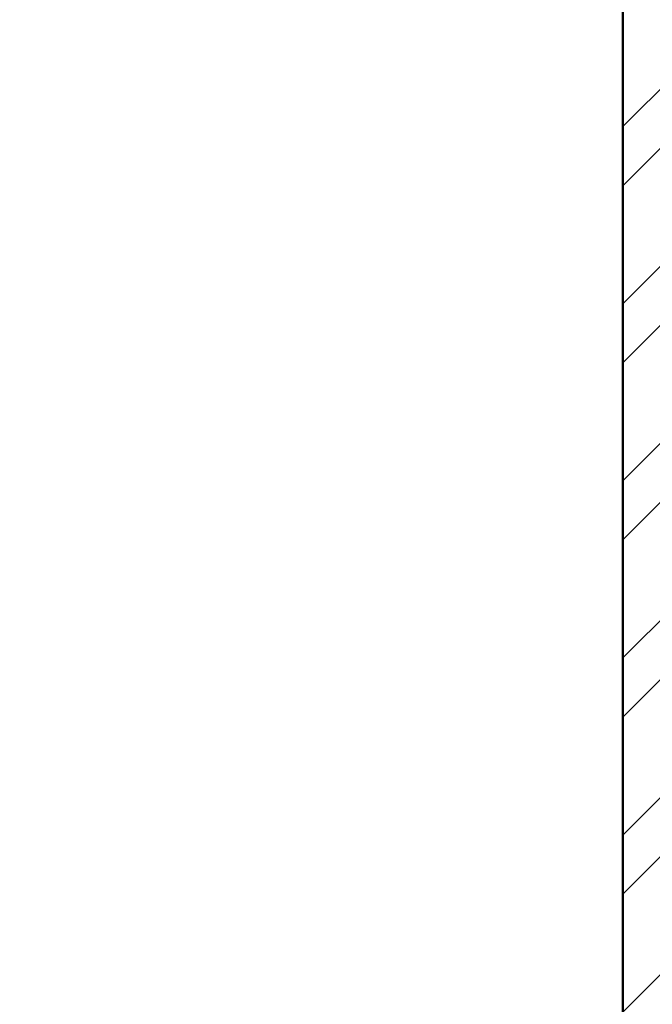
# Model space of a CAD drawing. Units: inches. Extents: x 1901 to 2863, y 888 to 2433.
# Tile 61 of 91: x 2121 to 2169, y 2127 to 2202. Entities that reach past the tile are written whole.
import ezdxf

# ---------------------------------------------------------------- set-up
doc = ezdxf.new("R2010")
doc.units = ezdxf.units.IN
doc.layers.add('A-WALL', color=7, linetype='Continuous', lineweight=50)
doc.layers.add('A-WALL-PATT', color=8, linetype='Continuous', lineweight=13)

msp = doc.modelspace()

# ---------------------------------------------------------------- hatches: boundary and pattern name
at = {"layer": 'A-WALL-PATT'}
h = msp.add_hatch(dxfattribs=at)
h.set_pattern_fill('ANSI32', color=256)
h.paths.add_polyline_path([(2192.501, 2274.134), (2141.264, 2274.134), (2141.264, 2269.634), (2192.501, 2269.634)])
h.paths.add_polyline_path([(2259.926, 2274.134), (2216.501, 2274.134), (2216.501, 2269.634), (2255.426, 2269.634), (2255.426, 2214.634), (2250.809, 2214.634), (2250.809, 2210.134), (2259.926, 2210.134), (2259.926, 2215.134), (2271.756, 2215.134), (2271.756, 2217.384), (2271.756, 2219.634), (2259.926, 2219.634)])
h.paths.add_polyline_path([(2171.426, 2269.634), (2166.926, 2269.634), (2166.926, 2219.634), (2121.238, 2219.634), (2121.238, 2215.134), (2166.926, 2215.134), (2166.926, 2083.134), (2161.807, 2083.134), (2161.807, 2078.634), (2171.426, 2078.634), (2176.996, 2078.634), (2176.996, 2080.884), (2176.996, 2083.134), (2171.426, 2083.134), (2171.426, 2210.134), (2230.912, 2210.134), (2230.912, 2212.384), (2230.912, 2214.634), (2171.426, 2214.634)])
h.paths.add_polyline_path([(2117.264, 2274.134), (2089.426, 2274.134), (2089.426, 2219.634), (2081.136, 2219.634), (2081.136, 2215.134), (2089.426, 2215.134), (2098.004, 2215.134), (2098.004, 2217.384), (2098.004, 2219.634), (2093.926, 2219.634), (2093.926, 2269.634), (2117.264, 2269.634), (2117.264, 2271.884)])
h.paths.add_polyline_path([(2343.426, 2219.634), (2329.295, 2219.634), (2329.295, 2215.134), (2338.926, 2215.134), (2338.926, 2184.739), (2343.426, 2184.739)])
h.paths.add_polyline_path([(2338.926, 2083.134), (2329.295, 2083.134), (2208.966, 2083.134), (2208.966, 2078.634), (2338.926, 2078.634)])
h.paths.add_polyline_path([(2343.426, 2136.739), (2338.926, 2136.739), (2338.926, 1872.634), (2343.426, 1872.634)])
h.paths.add_polyline_path([(2343.426, 1863.634), (2397.68, 1863.634), (2397.68, 1821.634), (2384.138, 1821.634), (2384.138, 1812.634), (2418.33, 1812.634), (2418.33, 1817.134), (2418.33, 1821.634), (2406.68, 1821.634), (2406.68, 1863.634), (2459.499, 1863.634), (2459.499, 1821.634), (2447.138, 1821.634), (2447.138, 1812.634), (2459.499, 1812.634), (2468.499, 1812.634), (2468.499, 1872.634), (2394.426, 1872.634), (2334.426, 1872.634), (2334.426, 1812.634), (2343.426, 1812.634), (2353.251, 1812.634), (2353.251, 1821.634), (2343.426, 1821.634)])
h.paths.add_polyline_path([(2510.014, 1872.634), (2468.499, 1872.634), (2468.499, 1868.134), (2510.014, 1868.134)])
h.paths.add_polyline_path([(2514.009, 1817.134), (2468.499, 1817.134), (2468.499, 1812.634), (2482.114, 1812.634), (2482.114, 1800.606), (2486.614, 1800.606), (2486.614, 1812.634), (2514.009, 1812.634)])
h.paths.add_polyline_path([(2299.247, 1814.884), (2299.247, 1817.134), (2295.926, 1817.134), (2295.926, 1854.169), (2293.676, 1854.169), (2291.426, 1854.169), (2291.426, 1817.134), (2266.109, 1817.134), (2266.109, 1812.634), (2299.247, 1812.634)])
h.paths.add_polyline_path([(2218.109, 1817.134), (2206.46, 1817.134), (2171.426, 1817.134), (2171.426, 1949.134), (2190.1, 1949.134), (2190.1, 1953.634), (2163.468, 1953.634), (2163.468, 1949.134), (2166.926, 1949.134), (2166.926, 1817.134), (2114.297, 1817.134), (2114.297, 1812.634), (2218.109, 1812.634)])
h.paths.add_polyline_path([(2029.426, 1970.922), (2024.926, 1970.922), (2024.926, 1912.717), (2029.426, 1912.717)])
h.paths.add_polyline_path([(2132.297, 1953.634), (2113.926, 1953.634), (2113.926, 1975.888), (2111.676, 1975.888), (2109.426, 1975.888), (2109.426, 1953.634), (2029.426, 1953.634), (2029.426, 1949.134), (2132.297, 1949.134)])
h.paths.add_polyline_path([(2029.426, 1853.606), (2029.31, 1853.606), (2029.31, 1853.606), (2029.426, 1853.606), (2029.426, 1864.717), (2024.926, 1864.717), (2024.926, 1812.634), (2066.297, 1812.634), (2066.297, 1814.884), (2066.297, 1817.134), (2029.426, 1817.134)])
h.paths.add_polyline_path([(2122.926, 2010.088), (2120.676, 2010.088), (2118.426, 2010.088), (2118.426, 2006.134), (2029.426, 2006.134), (2029.426, 2001.634), (2109.426, 2001.634), (2109.426, 1998.041), (2113.926, 1998.041), (2113.926, 2001.634), (2122.926, 2001.634)])
h.paths.add_polyline_path([(2029.426, 2031.376), (2024.926, 2031.376), (2024.926, 1994.922), (2027.176, 1994.922), (2029.426, 1994.922)])
h.paths.add_polyline_path([(2029.426, 2136.739), (2024.926, 2136.739), (2024.926, 2067.376), (2027.176, 2067.376), (2029.426, 2067.376)])
h.paths.add_polyline_path([(2125.618, 2083.134), (2029.426, 2083.134), (2029.426, 2078.634), (2118.426, 2078.634), (2118.426, 2030.715), (2122.926, 2030.715), (2122.926, 2078.634), (2125.618, 2078.634)])
h.paths.add_polyline_path([(2029.426, 2215.134), (2040.468, 2215.134), (2040.468, 2217.384), (2040.468, 2219.634), (2024.926, 2219.634), (2024.926, 2184.739), (2029.426, 2184.739), (2029.426, 2187.778)])
h.paths.add_polyline_path([(2686.426, 2274.134), (2659.284, 2274.134), (2659.284, 2269.634), (2681.926, 2269.634), (2681.926, 2219.634), (2676.816, 2219.634), (2676.816, 2215.134), (2681.926, 2215.134), (2697.011, 2215.134), (2697.011, 2217.384), (2697.011, 2219.634), (2686.426, 2219.634)])
h.paths.add_polyline_path([(2609.926, 2269.634), (2635.284, 2269.634), (2635.284, 2274.134), (2571.431, 2274.134), (2571.431, 2269.634), (2605.426, 2269.634), (2605.426, 2214.634), (2549.098, 2214.634), (2549.098, 2210.134), (2605.426, 2210.134), (2605.426, 2083.134), (2601.014, 2083.134), (2601.014, 2080.884), (2601.014, 2078.634), (2609.926, 2078.634), (2616.162, 2078.634), (2616.162, 2080.884), (2616.162, 2083.134), (2609.926, 2083.134), (2609.926, 2215.134), (2651.465, 2215.134), (2651.465, 2217.384), (2651.465, 2219.634), (2609.926, 2219.634)])
h.paths.add_polyline_path([(2521.426, 2269.634), (2547.431, 2269.634), (2547.431, 2271.884), (2547.431, 2274.134), (2516.926, 2274.134), (2516.926, 2219.634), (2506.41, 2219.634), (2506.41, 2215.134), (2516.926, 2215.134), (2516.926, 2210.134), (2525.402, 2210.134), (2525.402, 2212.384), (2525.402, 2214.634), (2521.426, 2214.634)])
h.paths.add_polyline_path([(2456.011, 2219.634), (2439.426, 2219.634), (2439.426, 2187.888), (2443.926, 2187.888), (2443.926, 2215.134), (2456.011, 2215.134)])
h.paths.add_polyline_path([(2752.926, 2219.634), (2739.485, 2219.634), (2739.485, 2215.134), (2748.426, 2215.134), (2748.426, 2187.888), (2752.926, 2187.888)])
h.paths.add_polyline_path([(2752.926, 2139.888), (2748.426, 2139.888), (2748.426, 2083.134), (2648.416, 2083.134), (2648.416, 2078.634), (2654.926, 2078.634), (2654.926, 2039.437), (2659.426, 2039.437), (2659.426, 2078.634), (2748.426, 2078.634), (2748.426, 2063.429), (2752.926, 2063.429)])
h.paths.add_polyline_path([(2752.926, 2010.634), (2659.426, 2010.634), (2659.426, 2015.652), (2654.926, 2015.652), (2654.926, 2010.634), (2605.426, 2010.634), (2605.426, 1920.967), (2609.926, 1920.967), (2609.926, 2006.134), (2748.426, 2006.134), (2748.426, 1982.466), (2752.926, 1982.466)])
h.paths.add_polyline_path([(2752.926, 2027.429), (2748.426, 2027.429), (2748.426, 2010.634), (2752.926, 2010.634)])
h.paths.add_polyline_path([(2748.426, 1886.134), (2609.926, 1886.134), (2609.926, 1889.719), (2605.426, 1889.719), (2605.426, 1861.262), (2609.926, 1861.262), (2609.926, 1881.634), (2748.426, 1881.634)])
h.paths.add_polyline_path([(2456.855, 2228.831), (2498.401, 2228.831), (2498.401, 2247.488), (2456.855, 2247.488)], flags=9)
h.paths.add_polyline_path([(2038.602, 2237.418), (2080.174, 2237.418), (2080.174, 2256.075), (2038.602, 2256.075)], flags=9)
h.paths.add_polyline_path([(2292.009, 1062.394), (2539.932, 1062.394), (2539.932, 1099.487), (2292.009, 1099.487)], flags=9)
h.paths.add_polyline_path([(2424.91, 1832.253), (2448.513, 1832.253), (2448.513, 1846.678), (2424.91, 1846.678)], flags=25)
h.paths.add_polyline_path([(2359.076, 1832.253), (2382.678, 1832.253), (2382.678, 1846.678), (2359.076, 1846.678)], flags=25)
h.paths.add_polyline_path([(2352.899, 1684.802), (2367.543, 1684.802), (2367.543, 1697.167), (2352.899, 1697.167)], flags=9)
h.paths.add_polyline_path([(2079.288, 1755.826), (2169.024, 1755.826), (2169.024, 1774.372), (2079.288, 1774.372)], flags=9)
h.paths.add_polyline_path([(2404.09, 1373.857), (2404.09, 1463.593), (2385.544, 1463.593), (2385.544, 1373.857)], flags=9)
h.paths.add_polyline_path([(2268.091, 2236.371), (2309.636, 2236.371), (2309.636, 2255.028), (2268.091, 2255.028)], flags=9)
h.paths.add_polyline_path([(2575.96, 1700.951), (2665.696, 1700.951), (2665.696, 1719.498), (2575.96, 1719.498)], flags=9)
h.paths.add_polyline_path([(2302.962, 1878.474), (2329.524, 1878.474), (2329.524, 1888.777), (2302.962, 1888.777)], flags=9)
h.paths.add_polyline_path([(2097.415, 2240.576), (2126.573, 2240.576), (2126.573, 2259.233), (2097.415, 2259.233)], flags=9)
h.paths.add_polyline_path([(2208.725, 2246.124), (2237.882, 2246.124), (2237.882, 2264.781), (2208.725, 2264.781)], flags=9)
h.paths.add_polyline_path([(2038.147, 1925.958), (2076.987, 1925.958), (2076.987, 1944.615), (2038.147, 1944.615)], flags=9)
h.paths.add_polyline_path([(2239.144, 1926.672), (2288.465, 1926.672), (2288.465, 1945.329), (2239.144, 1945.329)], flags=9)
h.paths.add_polyline_path([(2175.429, 2007.33), (2212.356, 2007.33), (2212.356, 2025.987), (2175.429, 2025.987)], flags=9)
h.paths.add_polyline_path([(2225.034, 2091.794), (2263.875, 2091.794), (2263.875, 2110.451), (2225.034, 2110.451)], flags=9)
h.paths.add_polyline_path([(2035.398, 2098.478), (2074.238, 2098.478), (2074.238, 2117.135), (2035.398, 2117.135)], flags=9)
h.paths.add_polyline_path([(2050.102, 2029.209), (2083.26, 2029.209), (2083.26, 2047.866), (2050.102, 2047.866)], flags=9)
h.paths.add_polyline_path([(2069.677, 1956.719), (2098.835, 1956.719), (2098.835, 1975.376), (2069.677, 1975.376)], flags=25)
h.paths.add_polyline_path([(2328.62, 1753.336), (2361.663, 1753.336), (2361.663, 1771.993), (2328.62, 1771.993)], flags=9)
h.paths.add_polyline_path([(2395.162, 2060.888), (2395.162, 2140.654), (2378.676, 2140.654), (2378.676, 2060.888)], flags=9)
h.paths.add_polyline_path([(2463.728, 2059.02), (2492.886, 2059.02), (2492.886, 2077.677), (2463.728, 2077.677)], flags=9)
h.paths.add_polyline_path([(2458.027, 2181.536), (2496.868, 2181.536), (2496.868, 2200.194), (2458.027, 2200.194)], flags=9)
h.paths.add_polyline_path([(2527.577, 2243.074), (2556.735, 2243.074), (2556.735, 2261.731), (2527.577, 2261.731)], flags=9)
h.paths.add_polyline_path([(2694.461, 2232.767), (2736.033, 2232.767), (2736.033, 2251.425), (2694.461, 2251.425)], flags=9)
h.paths.add_polyline_path([(2637.821, 2249.225), (2666.979, 2249.225), (2666.979, 2267.882), (2637.821, 2267.882)], flags=9)
h.paths.add_polyline_path([(2623.687, 2183.541), (2662.528, 2183.541), (2662.528, 2202.199), (2623.687, 2202.199)], flags=9)
h.paths.add_polyline_path([(2691.965, 2021.5), (2725.124, 2021.5), (2725.124, 2040.157), (2691.965, 2040.157)], flags=9)
h.paths.add_polyline_path([(2621.043, 1975.912), (2662.335, 1975.912), (2662.335, 1994.569), (2621.043, 1994.569)], flags=25)
h.paths.add_polyline_path([(2479.032, 1927.62), (2519.844, 1927.62), (2519.844, 1946.277), (2479.032, 1946.277)], flags=9)
h.paths.add_polyline_path([(2670.941, 1849.076), (2716.005, 1849.076), (2716.005, 1867.734), (2670.941, 1867.734)], flags=9)
h.paths.add_polyline_path([(2523.613, 1782.956), (2550.175, 1782.956), (2550.175, 1793.26), (2523.613, 1793.26)], flags=9)
h.paths.add_polyline_path([(2450.841, 1207.331), (2492.386, 1207.331), (2492.386, 1225.989), (2450.841, 1225.989)], flags=9)
h.paths.add_polyline_path([(2527.751, 1203.841), (2556.908, 1203.841), (2556.908, 1222.499), (2527.751, 1222.499)], flags=9)
h.paths.add_polyline_path([(2639.111, 1207.2), (2668.268, 1207.2), (2668.268, 1225.857), (2639.111, 1225.857)], flags=9)
h.paths.add_polyline_path([(2692.594, 1218.965), (2734.167, 1218.965), (2734.167, 1237.623), (2692.594, 1237.623)], flags=9)
h.paths.add_polyline_path([(2669.266, 1366.329), (2708.106, 1366.329), (2708.106, 1384.987), (2669.266, 1384.987)], flags=9)
h.paths.add_polyline_path([(2463.313, 1358.031), (2502.153, 1358.031), (2502.153, 1376.688), (2463.313, 1376.688)], flags=9)
h.paths.add_polyline_path([(2494.725, 1449.963), (2531.652, 1449.963), (2531.652, 1468.62), (2494.725, 1468.62)], flags=9)
h.paths.add_polyline_path([(2675.565, 1422.157), (2708.724, 1422.157), (2708.724, 1440.815), (2675.565, 1440.815)], flags=9)
h.paths.add_polyline_path([(2685.634, 1493.891), (2714.792, 1493.891), (2714.792, 1512.548), (2685.634, 1512.548)], flags=9)
h.paths.add_polyline_path([(2686.805, 1529.913), (2725.645, 1529.913), (2725.645, 1548.57), (2686.805, 1548.57)], flags=9)
h.paths.add_polyline_path([(2503.651, 1537.991), (2552.972, 1537.991), (2552.972, 1556.648), (2503.651, 1556.648)], flags=9)
h.paths.add_polyline_path([(2291.713, 1643.504), (2318.275, 1643.504), (2318.275, 1653.807), (2291.713, 1653.807)], flags=9)
h.paths.add_polyline_path([(2450.626, 1610.52), (2477.189, 1610.52), (2477.189, 1620.824), (2450.626, 1620.824)], flags=9)
h.paths.add_polyline_path([(2359.985, 1551.814), (2422.253, 1551.814), (2422.253, 1562.117), (2359.985, 1562.117)], flags=9)
h.paths.add_polyline_path([(2280.106, 1249.006), (2321.651, 1249.006), (2321.651, 1267.663), (2280.106, 1267.663)], flags=9)
h.paths.add_polyline_path([(2164.057, 1274.232), (2193.215, 1274.232), (2193.215, 1292.889), (2164.057, 1292.889)], flags=9)
h.paths.add_polyline_path([(2118.21, 1277.694), (2151.252, 1277.694), (2151.252, 1296.351), (2118.21, 1296.351)], flags=9)
h.paths.add_polyline_path([(2031.946, 1268.529), (2073.519, 1268.529), (2073.519, 1287.187), (2031.946, 1287.187)], flags=9)
h.paths.add_polyline_path([(2050.199, 1409.079), (2089.04, 1409.079), (2089.04, 1427.736), (2050.199, 1427.736)], flags=9)
h.paths.add_polyline_path([(2243.743, 1421.032), (2282.584, 1421.032), (2282.584, 1439.689), (2243.743, 1439.689)], flags=9)
h.paths.add_polyline_path([(2190.746, 1509.769), (2231.558, 1509.769), (2231.558, 1528.426), (2190.746, 1528.426)], flags=9)
h.paths.add_polyline_path([(2058.392, 1475.415), (2091.55, 1475.415), (2091.55, 1494.073), (2058.392, 1494.073)], flags=9)
h.paths.add_polyline_path([(2062.447, 1553.09), (2091.605, 1553.09), (2091.605, 1571.747), (2062.447, 1571.747)], flags=9)
h.paths.add_polyline_path([(2219.524, 1590.365), (2266.147, 1590.365), (2266.147, 1609.022), (2219.524, 1609.022)], flags=9)
h.paths.add_polyline_path([(2041.072, 1584.188), (2079.912, 1584.188), (2079.912, 1602.845), (2041.072, 1602.845)], flags=9)

# ---------------------------------------------------------------- linework, layer by layer
at = {"layer": 'A-WALL'}
msp.add_line((2166.926, 2215.134), (2166.926, 2083.134), dxfattribs=at)

doc.saveas('drawing.dxf')
